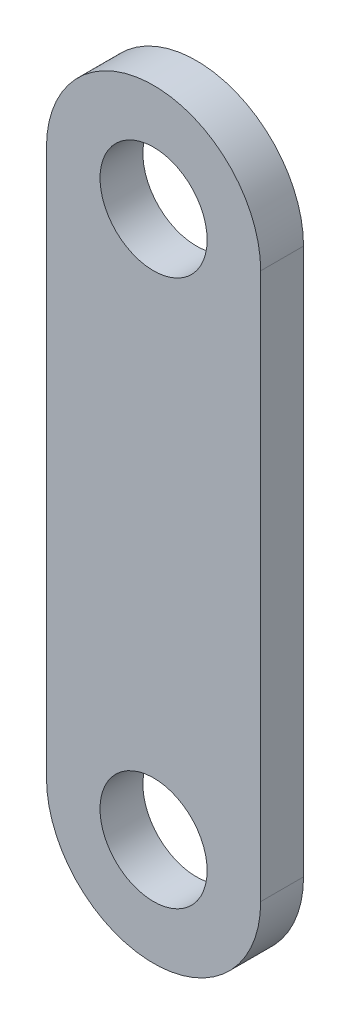
ISO-10303-21;
HEADER;
FILE_DESCRIPTION(('STEP AP214'),'2;1');
FILE_NAME('part.step','',(''),(''),'','','');
FILE_SCHEMA(('AUTOMOTIVE_DESIGN { 1 0 10303 214 1 1 1 1 }'));
ENDSEC;
DATA;
#1=APPLICATION_CONTEXT('core data for automotive mechanical design processes');
#2=APPLICATION_PROTOCOL_DEFINITION('international standard','automotive_design',2000,#1);
#3=PRODUCT_CONTEXT('',#1,'mechanical');
#4=PRODUCT('Part','Part','',(#3));
#5=PRODUCT_RELATED_PRODUCT_CATEGORY('part','',(#4));
#6=PRODUCT_DEFINITION_FORMATION('','',#4);
#7=PRODUCT_DEFINITION_CONTEXT('part definition',#1,'design');
#8=PRODUCT_DEFINITION('design','',#6,#7);
#9=PRODUCT_DEFINITION_SHAPE('','',#8);
#10=(LENGTH_UNIT() NAMED_UNIT(*) SI_UNIT(.MILLI.,.METRE.));
#11=(NAMED_UNIT(*) PLANE_ANGLE_UNIT() SI_UNIT($,.RADIAN.));
#12=(NAMED_UNIT(*) SI_UNIT($,.STERADIAN.) SOLID_ANGLE_UNIT());
#13=UNCERTAINTY_MEASURE_WITH_UNIT(LENGTH_MEASURE(1.E-05),#10,'distance_accuracy_value','');
#14=(GEOMETRIC_REPRESENTATION_CONTEXT(3) GLOBAL_UNCERTAINTY_ASSIGNED_CONTEXT((#13)) GLOBAL_UNIT_ASSIGNED_CONTEXT((#10,
#11,#12)) REPRESENTATION_CONTEXT('',''));
#15=CARTESIAN_POINT('',(0.,0.,0.));
#16=DIRECTION('',(0.,0.,1.));
#17=DIRECTION('',(1.,0.,0.));
#18=AXIS2_PLACEMENT_3D('',#15,#16,#17);
#19=CARTESIAN_POINT('',(0.,0.,20.));
#20=DIRECTION('',(0.,0.,1.));
#21=DIRECTION('',(1.,0.,0.));
#22=AXIS2_PLACEMENT_3D('',#19,#20,#21);
#23=PLANE('',#22);
#24=CARTESIAN_POINT('',(0.,255.,20.));
#25=DIRECTION('',(0.,0.,1.));
#26=DIRECTION('',(1.,0.,0.));
#27=AXIS2_PLACEMENT_3D('',#24,#25,#26);
#28=CIRCLE('',#27,25.);
#29=CARTESIAN_POINT('',(25.,255.,20.));
#30=VERTEX_POINT('',#29);
#31=EDGE_CURVE('E106',#30,#30,#28,.T.);
#32=ORIENTED_EDGE('',*,*,#31,.F.);
#33=EDGE_LOOP('',(#32));
#34=FACE_BOUND('',#33,.T.);
#35=CARTESIAN_POINT('',(0.,0.,20.));
#36=DIRECTION('',(0.,0.,1.));
#37=DIRECTION('',(1.,0.,0.));
#38=AXIS2_PLACEMENT_3D('',#35,#36,#37);
#39=CIRCLE('',#38,50.);
#40=CARTESIAN_POINT('',(-50.,0.,20.));
#41=VERTEX_POINT('',#40);
#42=CARTESIAN_POINT('',(50.,0.,20.));
#43=VERTEX_POINT('',#42);
#44=EDGE_CURVE('E93',#41,#43,#39,.T.);
#45=ORIENTED_EDGE('',*,*,#44,.T.);
#46=DIRECTION('',(0.,1.,0.));
#47=VECTOR('',#46,1.);
#48=CARTESIAN_POINT('',(50.,0.,20.));
#49=LINE('',#48,#47);
#50=CARTESIAN_POINT('',(50.,255.,20.));
#51=VERTEX_POINT('',#50);
#52=EDGE_CURVE('E88',#43,#51,#49,.T.);
#53=ORIENTED_EDGE('',*,*,#52,.T.);
#54=CARTESIAN_POINT('',(0.,255.,20.));
#55=DIRECTION('',(0.,0.,1.));
#56=DIRECTION('',(1.,0.,0.));
#57=AXIS2_PLACEMENT_3D('',#54,#55,#56);
#58=CIRCLE('',#57,50.);
#59=CARTESIAN_POINT('',(-50.,255.,20.));
#60=VERTEX_POINT('',#59);
#61=EDGE_CURVE('E90',#51,#60,#58,.T.);
#62=ORIENTED_EDGE('',*,*,#61,.T.);
#63=DIRECTION('',(0.,-1.,0.));
#64=VECTOR('',#63,1.);
#65=CARTESIAN_POINT('',(-50.,0.,20.));
#66=LINE('',#65,#64);
#67=EDGE_CURVE('E57',#60,#41,#66,.T.);
#68=ORIENTED_EDGE('',*,*,#67,.T.);
#69=EDGE_LOOP('',(#45,#53,#62,#68));
#70=FACE_BOUND('',#69,.T.);
#71=CARTESIAN_POINT('',(0.,0.,20.));
#72=DIRECTION('',(0.,0.,1.));
#73=DIRECTION('',(1.,0.,0.));
#74=AXIS2_PLACEMENT_3D('',#71,#72,#73);
#75=CIRCLE('',#74,25.);
#76=CARTESIAN_POINT('',(25.,0.,20.));
#77=VERTEX_POINT('',#76);
#78=EDGE_CURVE('E123',#77,#77,#75,.T.);
#79=ORIENTED_EDGE('',*,*,#78,.F.);
#80=EDGE_LOOP('',(#79));
#81=FACE_BOUND('',#80,.T.);
#82=ADVANCED_FACE('F39',(#34,#70,#81),#23,.T.);
#83=CARTESIAN_POINT('',(0.,0.,0.));
#84=DIRECTION('',(0.,0.,1.));
#85=DIRECTION('',(1.,0.,0.));
#86=AXIS2_PLACEMENT_3D('',#83,#84,#85);
#87=PLANE('',#86);
#88=CARTESIAN_POINT('',(0.,0.,0.));
#89=DIRECTION('',(0.,0.,1.));
#90=DIRECTION('',(1.,0.,0.));
#91=AXIS2_PLACEMENT_3D('',#88,#89,#90);
#92=CIRCLE('',#91,50.);
#93=CARTESIAN_POINT('',(-50.,0.,0.));
#94=VERTEX_POINT('',#93);
#95=CARTESIAN_POINT('',(50.,0.,0.));
#96=VERTEX_POINT('',#95);
#97=EDGE_CURVE('E103',#94,#96,#92,.T.);
#98=ORIENTED_EDGE('',*,*,#97,.F.);
#99=DIRECTION('',(0.,-1.,0.));
#100=VECTOR('',#99,1.);
#101=CARTESIAN_POINT('',(-50.,0.,0.));
#102=LINE('',#101,#100);
#103=CARTESIAN_POINT('',(-50.,255.,0.));
#104=VERTEX_POINT('',#103);
#105=EDGE_CURVE('E78',#104,#94,#102,.T.);
#106=ORIENTED_EDGE('',*,*,#105,.F.);
#107=CARTESIAN_POINT('',(0.,255.,0.));
#108=DIRECTION('',(0.,0.,1.));
#109=DIRECTION('',(1.,0.,0.));
#110=AXIS2_PLACEMENT_3D('',#107,#108,#109);
#111=CIRCLE('',#110,50.);
#112=CARTESIAN_POINT('',(50.,255.,0.));
#113=VERTEX_POINT('',#112);
#114=EDGE_CURVE('E71',#113,#104,#111,.T.);
#115=ORIENTED_EDGE('',*,*,#114,.F.);
#116=DIRECTION('',(0.,1.,0.));
#117=VECTOR('',#116,1.);
#118=CARTESIAN_POINT('',(50.,0.,0.));
#119=LINE('',#118,#117);
#120=EDGE_CURVE('E92',#96,#113,#119,.T.);
#121=ORIENTED_EDGE('',*,*,#120,.F.);
#122=EDGE_LOOP('',(#98,#106,#115,#121));
#123=FACE_BOUND('',#122,.T.);
#124=CARTESIAN_POINT('',(0.,255.,0.));
#125=DIRECTION('',(0.,0.,1.));
#126=DIRECTION('',(1.,0.,0.));
#127=AXIS2_PLACEMENT_3D('',#124,#125,#126);
#128=CIRCLE('',#127,25.);
#129=CARTESIAN_POINT('',(25.,255.,0.));
#130=VERTEX_POINT('',#129);
#131=EDGE_CURVE('E120',#130,#130,#128,.T.);
#132=ORIENTED_EDGE('',*,*,#131,.T.);
#133=EDGE_LOOP('',(#132));
#134=FACE_BOUND('',#133,.T.);
#135=CARTESIAN_POINT('',(0.,0.,0.));
#136=DIRECTION('',(0.,0.,1.));
#137=DIRECTION('',(1.,0.,0.));
#138=AXIS2_PLACEMENT_3D('',#135,#136,#137);
#139=CIRCLE('',#138,25.);
#140=CARTESIAN_POINT('',(25.,0.,0.));
#141=VERTEX_POINT('',#140);
#142=EDGE_CURVE('E125',#141,#141,#139,.T.);
#143=ORIENTED_EDGE('',*,*,#142,.T.);
#144=EDGE_LOOP('',(#143));
#145=FACE_BOUND('',#144,.T.);
#146=ADVANCED_FACE('F111',(#123,#134,#145),#87,.F.);
#147=CARTESIAN_POINT('',(0.,0.,20.));
#148=DIRECTION('',(0.,0.,-1.));
#149=DIRECTION('',(-1.,0.,0.));
#150=AXIS2_PLACEMENT_3D('',#147,#148,#149);
#151=CYLINDRICAL_SURFACE('',#150,50.);
#152=ORIENTED_EDGE('',*,*,#97,.T.);
#153=DIRECTION('',(0.,0.,-1.));
#154=VECTOR('',#153,1.);
#155=CARTESIAN_POINT('',(50.,0.,20.));
#156=LINE('',#155,#154);
#157=EDGE_CURVE('E11',#43,#96,#156,.T.);
#158=ORIENTED_EDGE('',*,*,#157,.F.);
#159=ORIENTED_EDGE('',*,*,#44,.F.);
#160=DIRECTION('',(0.,0.,-1.));
#161=VECTOR('',#160,1.);
#162=CARTESIAN_POINT('',(-50.,0.,20.));
#163=LINE('',#162,#161);
#164=EDGE_CURVE('E97',#41,#94,#163,.T.);
#165=ORIENTED_EDGE('',*,*,#164,.T.);
#166=EDGE_LOOP('',(#152,#158,#159,#165));
#167=FACE_BOUND('',#166,.T.);
#168=ADVANCED_FACE('F41',(#167),#151,.T.);
#169=CARTESIAN_POINT('',(50.,0.,20.));
#170=DIRECTION('',(-1.,0.,0.));
#171=DIRECTION('',(0.,0.,1.));
#172=AXIS2_PLACEMENT_3D('',#169,#170,#171);
#173=PLANE('',#172);
#174=ORIENTED_EDGE('',*,*,#120,.T.);
#175=DIRECTION('',(0.,0.,-1.));
#176=VECTOR('',#175,1.);
#177=CARTESIAN_POINT('',(50.,255.,20.));
#178=LINE('',#177,#176);
#179=EDGE_CURVE('E48',#51,#113,#178,.T.);
#180=ORIENTED_EDGE('',*,*,#179,.F.);
#181=ORIENTED_EDGE('',*,*,#52,.F.);
#182=ORIENTED_EDGE('',*,*,#157,.T.);
#183=EDGE_LOOP('',(#174,#180,#181,#182));
#184=FACE_BOUND('',#183,.T.);
#185=ADVANCED_FACE('F94',(#184),#173,.F.);
#186=CARTESIAN_POINT('',(0.,255.,20.));
#187=DIRECTION('',(0.,0.,-1.));
#188=DIRECTION('',(-1.,0.,0.));
#189=AXIS2_PLACEMENT_3D('',#186,#187,#188);
#190=CYLINDRICAL_SURFACE('',#189,50.);
#191=ORIENTED_EDGE('',*,*,#114,.T.);
#192=DIRECTION('',(0.,0.,-1.));
#193=VECTOR('',#192,1.);
#194=CARTESIAN_POINT('',(-50.,255.,20.));
#195=LINE('',#194,#193);
#196=EDGE_CURVE('E96',#60,#104,#195,.T.);
#197=ORIENTED_EDGE('',*,*,#196,.F.);
#198=ORIENTED_EDGE('',*,*,#61,.F.);
#199=ORIENTED_EDGE('',*,*,#179,.T.);
#200=EDGE_LOOP('',(#191,#197,#198,#199));
#201=FACE_BOUND('',#200,.T.);
#202=ADVANCED_FACE('F100',(#201),#190,.T.);
#203=CARTESIAN_POINT('',(-50.,0.,20.));
#204=DIRECTION('',(1.,0.,0.));
#205=DIRECTION('',(0.,0.,-1.));
#206=AXIS2_PLACEMENT_3D('',#203,#204,#205);
#207=PLANE('',#206);
#208=ORIENTED_EDGE('',*,*,#105,.T.);
#209=ORIENTED_EDGE('',*,*,#164,.F.);
#210=ORIENTED_EDGE('',*,*,#67,.F.);
#211=ORIENTED_EDGE('',*,*,#196,.T.);
#212=EDGE_LOOP('',(#208,#209,#210,#211));
#213=FACE_BOUND('',#212,.T.);
#214=ADVANCED_FACE('F112',(#213),#207,.F.);
#215=CARTESIAN_POINT('',(0.,255.,20.));
#216=DIRECTION('',(0.,0.,-1.));
#217=DIRECTION('',(-1.,0.,0.));
#218=AXIS2_PLACEMENT_3D('',#215,#216,#217);
#219=CYLINDRICAL_SURFACE('',#218,25.);
#220=ORIENTED_EDGE('',*,*,#31,.T.);
#221=EDGE_LOOP('',(#220));
#222=FACE_BOUND('',#221,.T.);
#223=ORIENTED_EDGE('',*,*,#131,.F.);
#224=EDGE_LOOP('',(#223));
#225=FACE_BOUND('',#224,.T.);
#226=ADVANCED_FACE('F143',(#222,#225),#219,.F.);
#227=CARTESIAN_POINT('',(0.,0.,20.));
#228=DIRECTION('',(0.,0.,-1.));
#229=DIRECTION('',(-1.,0.,0.));
#230=AXIS2_PLACEMENT_3D('',#227,#228,#229);
#231=CYLINDRICAL_SURFACE('',#230,25.);
#232=ORIENTED_EDGE('',*,*,#78,.T.);
#233=EDGE_LOOP('',(#232));
#234=FACE_BOUND('',#233,.T.);
#235=ORIENTED_EDGE('',*,*,#142,.F.);
#236=EDGE_LOOP('',(#235));
#237=FACE_BOUND('',#236,.T.);
#238=ADVANCED_FACE('F128',(#234,#237),#231,.F.);
#239=CLOSED_SHELL('',(#82,#146,#168,#185,#202,#214,#226,#238));
#240=MANIFOLD_SOLID_BREP('B2',#239);
#241=ADVANCED_BREP_SHAPE_REPRESENTATION('',(#18,#240),#14);
#242=SHAPE_DEFINITION_REPRESENTATION(#9,#241);
ENDSEC;
END-ISO-10303-21;
